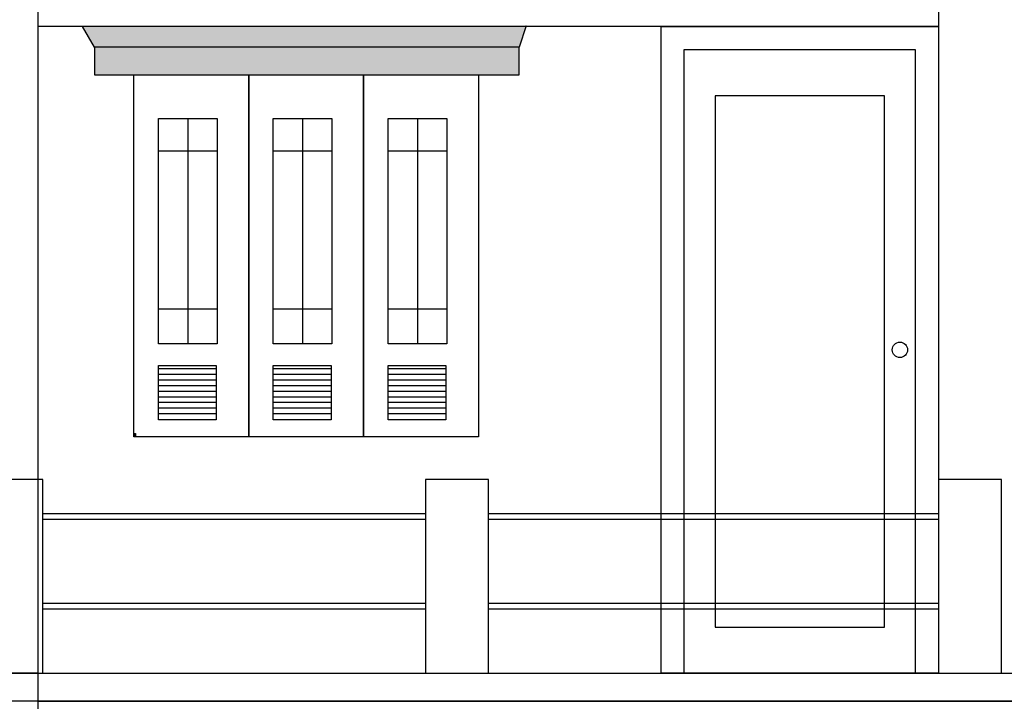
# Model space of a CAD drawing. Units: metres. Extents: x 10365 to 12529, y 3661 to 6248.
# Tile 7 of 9: x 11333 to 11858, y 5554 to 5918. Entities that reach past the tile are written whole.
import ezdxf

# ---------------------------------------------------------------- set-up
doc = ezdxf.new("R2010")
doc.units = ezdxf.units.M
doc.header["$MEASUREMENT"] = 0
doc.layers.add('A-ELEV', color=7, linetype='Continuous', lineweight=25)
doc.layers.add('A-ELEV-PATT', color=8, linetype='Continuous', lineweight=13)

# ---------------------------------------------------------------- blocks, each defined once
blk = doc.blocks.new('*U5')
blk.add_lwpolyline([(3, 0), (0, 0), (0, 72), (36, 72), (36, 0), (33, 0)])
for points in [[(33, 69), (33, 0), (3, 0), (3, 69)], [(29, 6), (29, 63), (7, 63), (7, 6)]]:
    blk.add_lwpolyline(points, close=True)
blk.add_circle((31, 42), 1)
blk = doc.blocks.new('*U6')
blk.add_lwpolyline([(3, 0), (0, 0), (0, 72), (36, 72), (36, 0), (33, 0)])
for points in [[(33, 69), (33, 0), (3, 0), (3, 69)], [(29, 6), (29, 63), (7, 63), (7, 6)]]:
    blk.add_lwpolyline(points, close=True)
blk.add_circle((31, 42), 1)
blk = doc.blocks.new('*U7')
blk.add_lwpolyline([(3.12, 0.01), (0.12, 0.01), (0.12, 84.01), (36.12, 84.01), (36.12, 0.01), (33.12, 0.01)])
for points in [[(33.12, 80.99), (33.12, 0.01), (3.12, 0.01), (3.12, 80.99)], [(29.12, 6.01), (29.12, 74.99), (7.12, 74.99), (7.12, 6.01)]]:
    blk.add_lwpolyline(points, close=True)
blk.add_circle((31.12, 42.01), 1)

msp = doc.modelspace()

# ---------------------------------------------------------------- hatches: boundary and pattern name
at = {"layer": 'A-ELEV-PATT'}
h = msp.add_hatch(color=256, dxfattribs=at)
h.dxf.hatch_style = 1
h.paths.add_polyline_path([(11599.63, 5903.01), (11373.23, 5903.01), (11373.23, 5888.32), (11599.63, 5888.32)])
h.paths.add_polyline_path([(11603.38, 5914.48), (11366.81, 5914.12), (11373.23, 5903.01), (11599.63, 5903.01)])

# ---------------------------------------------------------------- linework, layer by layer
at = {"layer": 'A-ELEV'}
for p, q in [((11343.22, 5554.17), (11343.22, 6116.31)), ((11823.22, 6116.31), (11823.22, 5604.54)), ((11823.22, 5914.12), (11343.22, 5914.12)), ((11366.81, 5914.12), (11603.38, 5914.48)), ((11373.23, 5903.01), (11366.81, 5914.12)), ((11603.38, 5914.48), (11599.63, 5903.01)), ((11422.93, 5865.03), (11422.93, 5744.86)), ((11484.2, 5865.03), (11484.2, 5744.86)), ((11545.46, 5865.03), (11545.46, 5744.86)), ((11407.32, 5847.66), (11438.55, 5847.66)), ((11468.58, 5847.66), (11499.81, 5847.66)), ((11529.85, 5847.66), (11561.07, 5847.66)), ((11407.32, 5763.45), (11438.55, 5763.45)), ((11468.58, 5763.45), (11499.81, 5763.45)), ((11529.85, 5763.45), (11561.07, 5763.45)), ((11407.32, 5731.63), (11438.08, 5731.63)), ((11407.32, 5728.63), (11438.08, 5728.63)), ((11468.58, 5731.63), (11499.34, 5731.63)), ((11468.58, 5728.63), (11499.34, 5728.63)), ((11529.85, 5731.63), (11560.6, 5731.63)), ((11529.85, 5728.63), (11560.6, 5728.63)), ((11407.32, 5725.63), (11438.08, 5725.63)), ((11407.32, 5722.63), (11438.08, 5722.63)), ((11468.58, 5725.63), (11499.34, 5725.63)), ((11468.58, 5722.63), (11499.34, 5722.63)), ((11529.85, 5725.63), (11560.6, 5725.63)), ((11529.85, 5722.63), (11560.6, 5722.63)), ((11407.32, 5719.63), (11438.08, 5719.63)), ((11468.58, 5719.63), (11499.34, 5719.63)), ((11529.85, 5719.63), (11560.6, 5719.63)), ((11407.32, 5716.63), (11438.08, 5716.63)), ((11407.32, 5713.63), (11438.08, 5713.63)), ((11407.32, 5713.63), (11438.08, 5713.63)), ((11468.58, 5716.63), (11499.34, 5716.63)), ((11468.58, 5713.63), (11499.34, 5713.63)), ((11468.58, 5713.63), (11499.34, 5713.63)), ((11529.85, 5716.63), (11560.6, 5716.63)), ((11529.85, 5713.63), (11560.6, 5713.63)), ((11529.85, 5713.63), (11560.6, 5713.63)), ((11407.32, 5710.63), (11438.08, 5710.63)), ((11407.32, 5707.63), (11438.08, 5707.63)), ((11468.58, 5710.63), (11499.34, 5710.63)), ((11468.58, 5707.63), (11499.34, 5707.63)), ((11529.85, 5710.63), (11560.6, 5710.63)), ((11529.85, 5707.63), (11560.6, 5707.63)), ((11345.66, 5654.29), (11549.69, 5654.29)), ((11345.66, 5651.29), (11549.69, 5651.29)), ((11583.32, 5654.29), (11823.22, 5654.29)), ((11583.32, 5651.29), (11823.22, 5651.29)), ((11345.66, 5606.51), (11549.69, 5606.51)), ((11345.66, 5603.51), (11549.69, 5603.51)), ((11583.32, 5606.51), (11823.22, 5606.51)), ((11583.32, 5603.51), (11823.22, 5603.51)), ((11343.22, 5569.17), (10563.57, 5569.17)), ((11343.22, 5569.17), (12303.22, 5569.17)), ((12303.22, 5554.17), (11343.22, 5554.17)), ((11343.22, 4875.44), (11343.22, 5554.17)), ((11343.22, 5554.17), (12303.22, 5554.17))]:
    msp.add_line(p, q, dxfattribs=at)
for points in [[(11373.23, 5888.32), (11373.23, 5888.32), (11599.63, 5888.32), (11599.63, 5888.32), (11599.63, 5903.01), (11599.63, 5903.01), (11373.23, 5903.01), (11373.23, 5903.01)], [(11394.2, 5888.32), (11394.2, 5888.32), (11455.47, 5888.32), (11455.47, 5888.32), (11455.47, 5695.23), (11455.47, 5695.23), (11394.2, 5695.23), (11394.2, 5695.23)], [(11455.47, 5888.32), (11455.47, 5888.32), (11516.73, 5888.32), (11516.73, 5888.32), (11516.73, 5695.23), (11516.73, 5695.23), (11455.47, 5695.23), (11455.47, 5695.23)], [(11516.73, 5888.32), (11516.73, 5888.32), (11577.99, 5888.32), (11577.99, 5888.32), (11577.99, 5695.23), (11577.99, 5695.23), (11516.73, 5695.23), (11516.73, 5695.23)], [(11407.32, 5865.03), (11407.32, 5865.03), (11438.55, 5865.03), (11438.55, 5865.03), (11438.55, 5744.86), (11438.55, 5744.86), (11407.32, 5744.86), (11407.32, 5744.86)], [(11468.58, 5865.03), (11468.58, 5865.03), (11499.81, 5865.03), (11499.81, 5865.03), (11499.81, 5744.86), (11499.81, 5744.86), (11468.58, 5744.86), (11468.58, 5744.86)], [(11529.85, 5865.03), (11529.85, 5865.03), (11561.07, 5865.03), (11561.07, 5865.03), (11561.07, 5744.86), (11561.07, 5744.86), (11529.85, 5744.86), (11529.85, 5744.86)], [(11407.32, 5733.31), (11407.32, 5733.31), (11438.08, 5733.31), (11438.08, 5733.31), (11438.08, 5704.34), (11438.08, 5704.34), (11407.32, 5704.34), (11407.32, 5704.34)], [(11468.58, 5733.31), (11468.58, 5733.31), (11499.34, 5733.31), (11499.34, 5733.31), (11499.34, 5704.34), (11499.34, 5704.34), (11468.58, 5704.34), (11468.58, 5704.34)], [(11529.85, 5733.31), (11529.85, 5733.31), (11560.6, 5733.31), (11560.6, 5733.31), (11560.6, 5704.34), (11560.6, 5704.34), (11529.85, 5704.34), (11529.85, 5704.34)], [(11312.04, 5569.17), (11312.04, 5569.17), (11345.66, 5569.17), (11345.66, 5569.17), (11345.66, 5672.53), (11345.66, 5672.53), (11312.04, 5672.53), (11312.04, 5672.53)], [(11549.69, 5569.17), (11549.69, 5569.17), (11583.32, 5569.17), (11583.32, 5569.17), (11583.32, 5672.53), (11583.32, 5672.53), (11549.69, 5672.53), (11549.69, 5672.53)], [(11823.22, 5569.17), (11823.22, 5569.17), (11856.84, 5569.17), (11856.84, 5569.17), (11856.84, 5672.53), (11856.84, 5672.53), (11823.22, 5672.53), (11823.22, 5672.53)], [(11343.22, 5554.17), (11343.22, 5554.17), (10590.74, 5554.17), (10590.74, 5554.17), (10590.74, 4925.82), (10590.74, 4925.82), (11343.22, 4925.82), (11343.22, 4925.82)]]:
    msp.add_lwpolyline(points, close=True, dxfattribs=at)

# ---------------------------------------------------------------- block references
for name, p, xscale, yscale, zscale in [('*U7', (11674.88, 5569.12), 4.106533305244322, 4.106533305244322, 4.106533305244322), ('*U5', (11394.2, 5695.23), 0.0254, 0.0254, 0.0254), ('*U6', (11394.2, 5695.23), 0.0254, 0.0254, 0.0254)]:
    msp.add_blockref(name, p, dxfattribs=dict(at, xscale=xscale, yscale=yscale, zscale=zscale))

doc.saveas('drawing.dxf')
